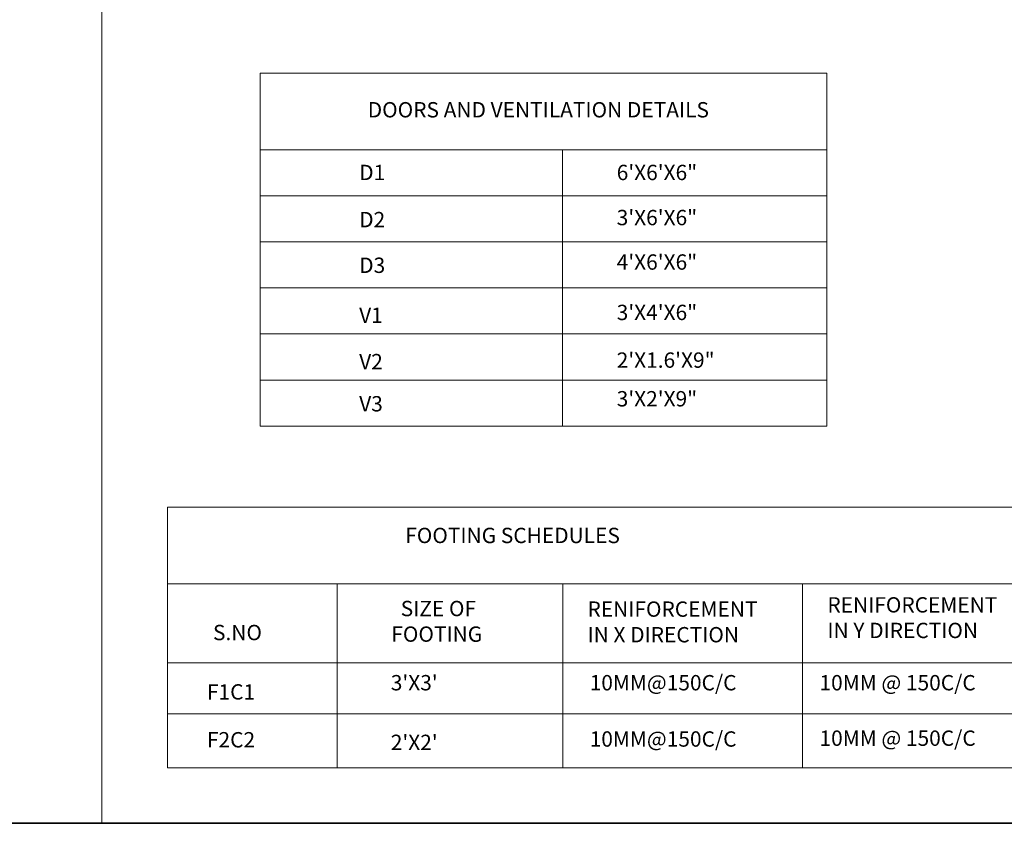
# Model space of a CAD drawing. Units: millimetres. Extents: x 20768 to 23556, y 50760 to 52704.
# Tile 7 of 36: x 21786 to 22556, y 50976 to 51604. Entities that reach past the tile are written whole.
import ezdxf

# ---------------------------------------------------------------- set-up
doc = ezdxf.new("R2010")
doc.units = ezdxf.units.MM
doc.layers.add('A-ANNO-SCHD', color=7, linetype='Continuous', lineweight=18)
doc.layers.add('A-ANNO-TTLB', color=7, linetype='Continuous', lineweight=35)
doc.styles.get("Standard").update_dxf_attribs({"font": 'arial.ttf'})

msp = doc.modelspace()

# ---------------------------------------------------------------- linework, layer by layer
at = {"layer": 'A-ANNO-SCHD'}
for p, q in [((21849.94, 51623.53), (21849.94, 50975.78)), ((21973.81, 51562.36), (22416.81, 51562.36)), ((21973.81, 51286.36), (21973.81, 51562.36)), ((22416.81, 51562.36), (22416.81, 51286.36)), ((21973.81, 51502.36), (22416.81, 51502.36)), ((22210.19, 51502.36), (22210.19, 51286.36)), ((21973.81, 51466.36), (22416.81, 51466.36)), ((21973.81, 51430.36), (22416.81, 51430.36)), ((21973.81, 51394.36), (22416.81, 51394.36)), ((21973.81, 51358.36), (22416.81, 51358.36)), ((21973.81, 51322.36), (22416.81, 51322.36)), ((21973.81, 51286.36), (22416.81, 51286.36)), ((21901.26, 51223.03), (22580.95, 51223.03)), ((21901.26, 51019.03), (21901.26, 51223.03)), ((21901.26, 51163.03), (22580.95, 51163.03)), ((22033.97, 51163.03), (22033.97, 51019.03)), ((22210.46, 51163.03), (22210.46, 51019.03)), ((22397.68, 51163.03), (22397.68, 51019.03)), ((21901.26, 51101.3), (22580.95, 51101.3)), ((21901.26, 51061.4), (22580.95, 51061.4)), ((21901.26, 51019.03), (22580.95, 51019.03))]:
    msp.add_line(p, q, dxfattribs=at)
at = {"layer": 'A-ANNO-TTLB'}
msp.add_line((20768.14, 50975.78), (22719.7, 50975.78), dxfattribs=at)

# ---------------------------------------------------------------- texts
at = {"layer": 'A-ANNO-SCHD', "char_height": 12, "attachment_point": 1}
for s, width, insert in [('DOORS AND VENTILATION DETAILS', 310.8077, (22057.85, 51539.67)), ('       D1', 80.0149, (22025.49, 51490.65)), ('      6\'X6\'X6"', 159.1438, (22230.52, 51490.65)), ('       D2', 80.0149, (22025.49, 51453.79)), ('      3\'X6\'X6"', 159.1438, (22230.52, 51455.39)), ('      4\'X6\'X6"', 159.1438, (22230.52, 51420.62)), ('       D3', 80.0149, (22025.49, 51418.08)), ('       V1', 80.0149, (22025.49, 51379)), ('      3\'X4\'X6"', 159.1438, (22230.52, 51381.22)), ('      2\'X1.6\'X9"', 159.1438, (22230.52, 51343.94)), ('       V2', 80.0149, (22025.49, 51342.75)), ('      3\'X2\'X9"', 159.1438, (22230.52, 51313.71)), ('       V3', 80.0149, (22025.49, 51309.8)), ('        FOOTING SCHEDULES', 310.8077, (22057.85, 51206.85)), ('RENIFORCEMENT \\PIN Y DIRECTION', 157.107, (22417.28, 51152.58)), ('    SIZE OF \\P  FOOTING', 125.9936, (22068.96, 51149.71)), ('RENIFORCEMENT \\PIN X DIRECTION', 157.107, (22229.7, 51149.25)), ('     S.NO', 80.0149, (21918.53, 51130.95)), ("      3'X3'", 159.1438, (22053.88, 51091.71)), ('      10MM@150C/C', 159.1438, (22209.38, 51091.71)), ('      10MM @ 150C/C', 159.1438, (22389.09, 51091.71)), ('    F1C1', 80.0149, (21917.47, 51084.53)), ('    F2C2', 80.0149, (21917.47, 51047.12)), ("      2'X2'", 159.1438, (22053.88, 51045.07)), ('      10MM@150C/C', 159.1438, (22209.38, 51047.7)), ('      10MM @ 150C/C', 159.1438, (22389.09, 51048.35))]:
    msp.add_mtext_dynamic_manual_height_columns(s, width=width, gutter_width=12.5, heights=[0], dxfattribs=dict(at, insert=insert))

doc.saveas('drawing.dxf')
